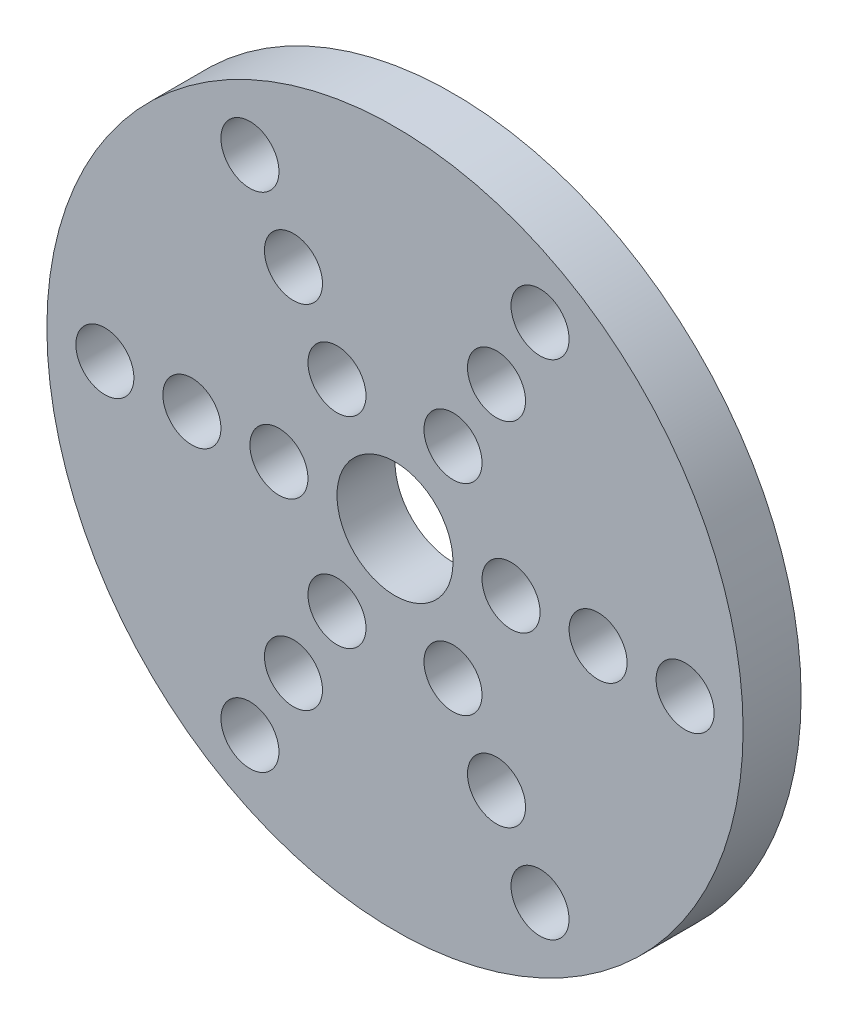
ISO-10303-21;
HEADER;
FILE_DESCRIPTION(('STEP AP214'),'2;1');
FILE_NAME('part.step','',(''),(''),'','','');
FILE_SCHEMA(('AUTOMOTIVE_DESIGN { 1 0 10303 214 1 1 1 1 }'));
ENDSEC;
DATA;
#1=APPLICATION_CONTEXT('core data for automotive mechanical design processes');
#2=APPLICATION_PROTOCOL_DEFINITION('international standard','automotive_design',2000,#1);
#3=PRODUCT_CONTEXT('',#1,'mechanical');
#4=PRODUCT('Part','Part','',(#3));
#5=PRODUCT_RELATED_PRODUCT_CATEGORY('part','',(#4));
#6=PRODUCT_DEFINITION_FORMATION('','',#4);
#7=PRODUCT_DEFINITION_CONTEXT('part definition',#1,'design');
#8=PRODUCT_DEFINITION('design','',#6,#7);
#9=PRODUCT_DEFINITION_SHAPE('','',#8);
#10=(LENGTH_UNIT() NAMED_UNIT(*) SI_UNIT(.MILLI.,.METRE.));
#11=(NAMED_UNIT(*) PLANE_ANGLE_UNIT() SI_UNIT($,.RADIAN.));
#12=(NAMED_UNIT(*) SI_UNIT($,.STERADIAN.) SOLID_ANGLE_UNIT());
#13=UNCERTAINTY_MEASURE_WITH_UNIT(LENGTH_MEASURE(1.E-05),#10,'distance_accuracy_value','');
#14=(GEOMETRIC_REPRESENTATION_CONTEXT(3) GLOBAL_UNCERTAINTY_ASSIGNED_CONTEXT((#13)) GLOBAL_UNIT_ASSIGNED_CONTEXT((#10,
#11,#12)) REPRESENTATION_CONTEXT('',''));
#15=CARTESIAN_POINT('',(0.,0.,0.));
#16=DIRECTION('',(0.,0.,1.));
#17=DIRECTION('',(1.,0.,0.));
#18=AXIS2_PLACEMENT_3D('',#15,#16,#17);
#19=CARTESIAN_POINT('',(0.,0.,10.));
#20=DIRECTION('',(0.,0.,-1.));
#21=DIRECTION('',(-1.,0.,0.));
#22=AXIS2_PLACEMENT_3D('',#19,#20,#21);
#23=CYLINDRICAL_SURFACE('',#22,60.);
#24=CARTESIAN_POINT('',(0.,0.,10.));
#25=DIRECTION('',(0.,0.,1.));
#26=DIRECTION('',(1.,0.,0.));
#27=AXIS2_PLACEMENT_3D('',#24,#25,#26);
#28=CIRCLE('',#27,60.);
#29=CARTESIAN_POINT('',(60.,0.,10.));
#30=VERTEX_POINT('',#29);
#31=EDGE_CURVE('E10',#30,#30,#28,.T.);
#32=ORIENTED_EDGE('',*,*,#31,.F.);
#33=EDGE_LOOP('',(#32));
#34=FACE_BOUND('',#33,.T.);
#35=CARTESIAN_POINT('',(0.,0.,0.));
#36=DIRECTION('',(0.,0.,1.));
#37=DIRECTION('',(1.,0.,0.));
#38=AXIS2_PLACEMENT_3D('',#35,#36,#37);
#39=CIRCLE('',#38,60.);
#40=CARTESIAN_POINT('',(60.,0.,0.));
#41=VERTEX_POINT('',#40);
#42=EDGE_CURVE('E45',#41,#41,#39,.T.);
#43=ORIENTED_EDGE('',*,*,#42,.T.);
#44=EDGE_LOOP('',(#43));
#45=FACE_BOUND('',#44,.T.);
#46=ADVANCED_FACE('F39',(#34,#45),#23,.T.);
#47=CARTESIAN_POINT('',(0.,0.,10.));
#48=DIRECTION('',(0.,0.,1.));
#49=DIRECTION('',(1.,0.,0.));
#50=AXIS2_PLACEMENT_3D('',#47,#48,#49);
#51=PLANE('',#50);
#52=CARTESIAN_POINT('',(17.5000000000004,30.3108891324552,10.));
#53=DIRECTION('',(0.,0.,1.));
#54=DIRECTION('',(0.50000000000001,0.866025403784433,0.));
#55=AXIS2_PLACEMENT_3D('',#52,#53,#54);
#56=CIRCLE('',#55,5.);
#57=CARTESIAN_POINT('',(20.0000000000004,34.6410161513773,10.));
#58=VERTEX_POINT('',#57);
#59=EDGE_CURVE('E157',#58,#58,#56,.T.);
#60=ORIENTED_EDGE('',*,*,#59,.F.);
#61=EDGE_LOOP('',(#60));
#62=FACE_BOUND('',#61,.T.);
#63=CARTESIAN_POINT('',(25.0000000000005,43.3012701892216,10.));
#64=DIRECTION('',(0.,0.,1.));
#65=DIRECTION('',(0.50000000000001,0.866025403784433,0.));
#66=AXIS2_PLACEMENT_3D('',#63,#64,#65);
#67=CIRCLE('',#66,5.);
#68=CARTESIAN_POINT('',(27.5000000000006,47.6313972081438,10.));
#69=VERTEX_POINT('',#68);
#70=EDGE_CURVE('E153',#69,#69,#67,.T.);
#71=ORIENTED_EDGE('',*,*,#70,.F.);
#72=EDGE_LOOP('',(#71));
#73=FACE_BOUND('',#72,.T.);
#74=CARTESIAN_POINT('',(-17.4999999999997,30.3108891324555,10.));
#75=DIRECTION('',(0.,0.,1.));
#76=DIRECTION('',(-0.499999999999992,0.866025403784443,0.));
#77=AXIS2_PLACEMENT_3D('',#74,#75,#76);
#78=CIRCLE('',#77,5.);
#79=CARTESIAN_POINT('',(-19.9999999999997,34.6410161513777,10.));
#80=VERTEX_POINT('',#79);
#81=EDGE_CURVE('E146',#80,#80,#78,.T.);
#82=ORIENTED_EDGE('',*,*,#81,.F.);
#83=EDGE_LOOP('',(#82));
#84=FACE_BOUND('',#83,.T.);
#85=CARTESIAN_POINT('',(-24.9999999999996,43.3012701892222,10.));
#86=DIRECTION('',(0.,0.,1.));
#87=DIRECTION('',(-0.499999999999992,0.866025403784443,0.));
#88=AXIS2_PLACEMENT_3D('',#85,#86,#87);
#89=CIRCLE('',#88,5.);
#90=CARTESIAN_POINT('',(-27.4999999999996,47.6313972081444,10.));
#91=VERTEX_POINT('',#90);
#92=EDGE_CURVE('E143',#91,#91,#89,.T.);
#93=ORIENTED_EDGE('',*,*,#92,.F.);
#94=EDGE_LOOP('',(#93));
#95=FACE_BOUND('',#94,.T.);
#96=CARTESIAN_POINT('',(-35.,0.,10.));
#97=DIRECTION('',(0.,0.,1.));
#98=DIRECTION('',(-1.,0.,0.));
#99=AXIS2_PLACEMENT_3D('',#96,#97,#98);
#100=CIRCLE('',#99,5.);
#101=CARTESIAN_POINT('',(-40.,0.,10.));
#102=VERTEX_POINT('',#101);
#103=EDGE_CURVE('E138',#102,#102,#100,.T.);
#104=ORIENTED_EDGE('',*,*,#103,.F.);
#105=EDGE_LOOP('',(#104));
#106=FACE_BOUND('',#105,.T.);
#107=CARTESIAN_POINT('',(-50.,0.,10.));
#108=DIRECTION('',(0.,0.,1.));
#109=DIRECTION('',(-1.,0.,0.));
#110=AXIS2_PLACEMENT_3D('',#107,#108,#109);
#111=CIRCLE('',#110,5.);
#112=CARTESIAN_POINT('',(-55.,0.,10.));
#113=VERTEX_POINT('',#112);
#114=EDGE_CURVE('E129',#113,#113,#111,.T.);
#115=ORIENTED_EDGE('',*,*,#114,.F.);
#116=EDGE_LOOP('',(#115));
#117=FACE_BOUND('',#116,.T.);
#118=CARTESIAN_POINT('',(-17.5000000000001,-30.3108891324553,10.));
#119=DIRECTION('',(0.,0.,1.));
#120=DIRECTION('',(-0.500000000000004,-0.866025403784436,0.));
#121=AXIS2_PLACEMENT_3D('',#118,#119,#120);
#122=CIRCLE('',#121,5.);
#123=CARTESIAN_POINT('',(-20.0000000000002,-34.6410161513775,10.));
#124=VERTEX_POINT('',#123);
#125=EDGE_CURVE('E122',#124,#124,#122,.T.);
#126=ORIENTED_EDGE('',*,*,#125,.F.);
#127=EDGE_LOOP('',(#126));
#128=FACE_BOUND('',#127,.T.);
#129=CARTESIAN_POINT('',(-25.0000000000002,-43.3012701892218,10.));
#130=DIRECTION('',(0.,0.,1.));
#131=DIRECTION('',(-0.500000000000004,-0.866025403784436,0.));
#132=AXIS2_PLACEMENT_3D('',#129,#130,#131);
#133=CIRCLE('',#132,5.);
#134=CARTESIAN_POINT('',(-27.5000000000002,-47.631397208144,10.));
#135=VERTEX_POINT('',#134);
#136=EDGE_CURVE('E119',#135,#135,#133,.T.);
#137=ORIENTED_EDGE('',*,*,#136,.F.);
#138=EDGE_LOOP('',(#137));
#139=FACE_BOUND('',#138,.T.);
#140=CARTESIAN_POINT('',(17.4999999999999,-30.3108891324554,10.));
#141=DIRECTION('',(0.,0.,1.));
#142=DIRECTION('',(0.499999999999998,-0.86602540378444,0.));
#143=AXIS2_PLACEMENT_3D('',#140,#141,#142);
#144=CIRCLE('',#143,5.);
#145=CARTESIAN_POINT('',(19.9999999999999,-34.6410161513776,10.));
#146=VERTEX_POINT('',#145);
#147=EDGE_CURVE('E115',#146,#146,#144,.T.);
#148=ORIENTED_EDGE('',*,*,#147,.F.);
#149=EDGE_LOOP('',(#148));
#150=FACE_BOUND('',#149,.T.);
#151=CARTESIAN_POINT('',(24.9999999999999,-43.301270189222,10.));
#152=DIRECTION('',(0.,0.,1.));
#153=DIRECTION('',(0.499999999999998,-0.86602540378444,0.));
#154=AXIS2_PLACEMENT_3D('',#151,#152,#153);
#155=CIRCLE('',#154,5.);
#156=CARTESIAN_POINT('',(27.4999999999999,-47.6313972081442,10.));
#157=VERTEX_POINT('',#156);
#158=EDGE_CURVE('E104',#157,#157,#155,.T.);
#159=ORIENTED_EDGE('',*,*,#158,.F.);
#160=EDGE_LOOP('',(#159));
#161=FACE_BOUND('',#160,.T.);
#162=CARTESIAN_POINT('',(35.,0.,10.));
#163=DIRECTION('',(0.,0.,1.));
#164=DIRECTION('',(1.,0.,0.));
#165=AXIS2_PLACEMENT_3D('',#162,#163,#164);
#166=CIRCLE('',#165,5.);
#167=CARTESIAN_POINT('',(40.,0.,10.));
#168=VERTEX_POINT('',#167);
#169=EDGE_CURVE('E99',#168,#168,#166,.T.);
#170=ORIENTED_EDGE('',*,*,#169,.F.);
#171=EDGE_LOOP('',(#170));
#172=FACE_BOUND('',#171,.T.);
#173=CARTESIAN_POINT('',(50.,0.,10.));
#174=DIRECTION('',(0.,0.,1.));
#175=DIRECTION('',(1.,0.,0.));
#176=AXIS2_PLACEMENT_3D('',#173,#174,#175);
#177=CIRCLE('',#176,5.);
#178=CARTESIAN_POINT('',(55.,0.,10.));
#179=VERTEX_POINT('',#178);
#180=EDGE_CURVE('E91',#179,#179,#177,.T.);
#181=ORIENTED_EDGE('',*,*,#180,.F.);
#182=EDGE_LOOP('',(#181));
#183=FACE_BOUND('',#182,.T.);
#184=CARTESIAN_POINT('',(10.0000000000002,17.3205080756887,10.));
#185=DIRECTION('',(0.,0.,1.));
#186=DIRECTION('',(0.50000000000001,0.866025403784433,0.));
#187=AXIS2_PLACEMENT_3D('',#184,#185,#186);
#188=CIRCLE('',#187,5.);
#189=CARTESIAN_POINT('',(12.5000000000003,21.6506350946108,10.));
#190=VERTEX_POINT('',#189);
#191=EDGE_CURVE('E67',#190,#190,#188,.T.);
#192=ORIENTED_EDGE('',*,*,#191,.F.);
#193=EDGE_LOOP('',(#192));
#194=FACE_BOUND('',#193,.T.);
#195=CARTESIAN_POINT('',(-9.99999999999984,17.3205080756889,10.));
#196=DIRECTION('',(0.,0.,1.));
#197=DIRECTION('',(-0.499999999999992,0.866025403784443,0.));
#198=AXIS2_PLACEMENT_3D('',#195,#196,#197);
#199=CIRCLE('',#198,5.);
#200=CARTESIAN_POINT('',(-12.4999999999998,21.6506350946111,10.));
#201=VERTEX_POINT('',#200);
#202=EDGE_CURVE('E78',#201,#201,#199,.T.);
#203=ORIENTED_EDGE('',*,*,#202,.F.);
#204=EDGE_LOOP('',(#203));
#205=FACE_BOUND('',#204,.T.);
#206=CARTESIAN_POINT('',(-20.,0.,10.));
#207=DIRECTION('',(0.,0.,1.));
#208=DIRECTION('',(-1.,0.,0.));
#209=AXIS2_PLACEMENT_3D('',#206,#207,#208);
#210=CIRCLE('',#209,5.);
#211=CARTESIAN_POINT('',(-25.,0.,10.));
#212=VERTEX_POINT('',#211);
#213=EDGE_CURVE('E85',#212,#212,#210,.T.);
#214=ORIENTED_EDGE('',*,*,#213,.F.);
#215=EDGE_LOOP('',(#214));
#216=FACE_BOUND('',#215,.T.);
#217=CARTESIAN_POINT('',(-10.0000000000001,-17.3205080756887,10.));
#218=DIRECTION('',(0.,0.,1.));
#219=DIRECTION('',(-0.500000000000004,-0.866025403784436,0.));
#220=AXIS2_PLACEMENT_3D('',#217,#218,#219);
#221=CIRCLE('',#220,5.);
#222=CARTESIAN_POINT('',(-12.5000000000001,-21.6506350946109,10.));
#223=VERTEX_POINT('',#222);
#224=EDGE_CURVE('E86',#223,#223,#221,.T.);
#225=ORIENTED_EDGE('',*,*,#224,.F.);
#226=EDGE_LOOP('',(#225));
#227=FACE_BOUND('',#226,.T.);
#228=CARTESIAN_POINT('',(9.99999999999996,-17.3205080756888,10.));
#229=DIRECTION('',(0.,0.,1.));
#230=DIRECTION('',(0.499999999999998,-0.86602540378444,0.));
#231=AXIS2_PLACEMENT_3D('',#228,#229,#230);
#232=CIRCLE('',#231,5.);
#233=CARTESIAN_POINT('',(12.5,-21.650635094611,10.));
#234=VERTEX_POINT('',#233);
#235=EDGE_CURVE('E62',#234,#234,#232,.T.);
#236=ORIENTED_EDGE('',*,*,#235,.F.);
#237=EDGE_LOOP('',(#236));
#238=FACE_BOUND('',#237,.T.);
#239=CARTESIAN_POINT('',(20.,0.,10.));
#240=DIRECTION('',(0.,0.,1.));
#241=DIRECTION('',(1.,0.,0.));
#242=AXIS2_PLACEMENT_3D('',#239,#240,#241);
#243=CIRCLE('',#242,5.);
#244=CARTESIAN_POINT('',(25.,0.,10.));
#245=VERTEX_POINT('',#244);
#246=EDGE_CURVE('E60',#245,#245,#243,.T.);
#247=ORIENTED_EDGE('',*,*,#246,.F.);
#248=EDGE_LOOP('',(#247));
#249=FACE_BOUND('',#248,.T.);
#250=CARTESIAN_POINT('',(0.,0.,10.));
#251=DIRECTION('',(0.,0.,1.));
#252=DIRECTION('',(1.,0.,0.));
#253=AXIS2_PLACEMENT_3D('',#250,#251,#252);
#254=CIRCLE('',#253,10.);
#255=CARTESIAN_POINT('',(10.,0.,10.));
#256=VERTEX_POINT('',#255);
#257=EDGE_CURVE('E51',#256,#256,#254,.T.);
#258=ORIENTED_EDGE('',*,*,#257,.F.);
#259=EDGE_LOOP('',(#258));
#260=FACE_BOUND('',#259,.T.);
#261=ORIENTED_EDGE('',*,*,#31,.T.);
#262=EDGE_LOOP('',(#261));
#263=FACE_BOUND('',#262,.T.);
#264=ADVANCED_FACE('F171',(#62,#73,#84,#95,#106,#117,#128,#139,#150,#161,#172,#183,#194,#205,
#216,#227,#238,#249,#260,#263),#51,.T.);
#265=CARTESIAN_POINT('',(0.,0.,0.));
#266=DIRECTION('',(0.,0.,1.));
#267=DIRECTION('',(1.,0.,0.));
#268=AXIS2_PLACEMENT_3D('',#265,#266,#267);
#269=PLANE('',#268);
#270=CARTESIAN_POINT('',(17.5000000000004,30.3108891324552,0.));
#271=DIRECTION('',(0.,0.,1.));
#272=DIRECTION('',(0.50000000000001,0.866025403784433,0.));
#273=AXIS2_PLACEMENT_3D('',#270,#271,#272);
#274=CIRCLE('',#273,5.);
#275=CARTESIAN_POINT('',(20.0000000000004,34.6410161513773,0.));
#276=VERTEX_POINT('',#275);
#277=EDGE_CURVE('E144',#276,#276,#274,.T.);
#278=ORIENTED_EDGE('',*,*,#277,.T.);
#279=EDGE_LOOP('',(#278));
#280=FACE_BOUND('',#279,.T.);
#281=CARTESIAN_POINT('',(25.0000000000005,43.3012701892216,0.));
#282=DIRECTION('',(0.,0.,1.));
#283=DIRECTION('',(0.50000000000001,0.866025403784433,0.));
#284=AXIS2_PLACEMENT_3D('',#281,#282,#283);
#285=CIRCLE('',#284,5.);
#286=CARTESIAN_POINT('',(27.5000000000006,47.6313972081438,0.));
#287=VERTEX_POINT('',#286);
#288=EDGE_CURVE('E156',#287,#287,#285,.T.);
#289=ORIENTED_EDGE('',*,*,#288,.T.);
#290=EDGE_LOOP('',(#289));
#291=FACE_BOUND('',#290,.T.);
#292=CARTESIAN_POINT('',(-17.4999999999997,30.3108891324555,0.));
#293=DIRECTION('',(0.,0.,1.));
#294=DIRECTION('',(-0.499999999999992,0.866025403784443,0.));
#295=AXIS2_PLACEMENT_3D('',#292,#293,#294);
#296=CIRCLE('',#295,5.);
#297=CARTESIAN_POINT('',(-19.9999999999997,34.6410161513777,0.));
#298=VERTEX_POINT('',#297);
#299=EDGE_CURVE('E132',#298,#298,#296,.T.);
#300=ORIENTED_EDGE('',*,*,#299,.T.);
#301=EDGE_LOOP('',(#300));
#302=FACE_BOUND('',#301,.T.);
#303=CARTESIAN_POINT('',(-24.9999999999996,43.3012701892222,0.));
#304=DIRECTION('',(0.,0.,1.));
#305=DIRECTION('',(-0.499999999999992,0.866025403784443,0.));
#306=AXIS2_PLACEMENT_3D('',#303,#304,#305);
#307=CIRCLE('',#306,5.);
#308=CARTESIAN_POINT('',(-27.4999999999996,47.6313972081444,0.));
#309=VERTEX_POINT('',#308);
#310=EDGE_CURVE('E145',#309,#309,#307,.T.);
#311=ORIENTED_EDGE('',*,*,#310,.T.);
#312=EDGE_LOOP('',(#311));
#313=FACE_BOUND('',#312,.T.);
#314=CARTESIAN_POINT('',(-35.,0.,0.));
#315=DIRECTION('',(0.,0.,1.));
#316=DIRECTION('',(-1.,0.,0.));
#317=AXIS2_PLACEMENT_3D('',#314,#315,#316);
#318=CIRCLE('',#317,5.);
#319=CARTESIAN_POINT('',(-40.,0.,0.));
#320=VERTEX_POINT('',#319);
#321=EDGE_CURVE('E123',#320,#320,#318,.T.);
#322=ORIENTED_EDGE('',*,*,#321,.T.);
#323=EDGE_LOOP('',(#322));
#324=FACE_BOUND('',#323,.T.);
#325=CARTESIAN_POINT('',(-50.,0.,0.));
#326=DIRECTION('',(0.,0.,1.));
#327=DIRECTION('',(-1.,0.,0.));
#328=AXIS2_PLACEMENT_3D('',#325,#326,#327);
#329=CIRCLE('',#328,5.);
#330=CARTESIAN_POINT('',(-55.,0.,0.));
#331=VERTEX_POINT('',#330);
#332=EDGE_CURVE('E134',#331,#331,#329,.T.);
#333=ORIENTED_EDGE('',*,*,#332,.T.);
#334=EDGE_LOOP('',(#333));
#335=FACE_BOUND('',#334,.T.);
#336=CARTESIAN_POINT('',(-17.5000000000001,-30.3108891324553,0.));
#337=DIRECTION('',(0.,0.,1.));
#338=DIRECTION('',(-0.500000000000004,-0.866025403784436,0.));
#339=AXIS2_PLACEMENT_3D('',#336,#337,#338);
#340=CIRCLE('',#339,5.);
#341=CARTESIAN_POINT('',(-20.0000000000002,-34.6410161513775,0.));
#342=VERTEX_POINT('',#341);
#343=EDGE_CURVE('E108',#342,#342,#340,.T.);
#344=ORIENTED_EDGE('',*,*,#343,.T.);
#345=EDGE_LOOP('',(#344));
#346=FACE_BOUND('',#345,.T.);
#347=CARTESIAN_POINT('',(-25.0000000000002,-43.3012701892218,0.));
#348=DIRECTION('',(0.,0.,1.));
#349=DIRECTION('',(-0.500000000000004,-0.866025403784436,0.));
#350=AXIS2_PLACEMENT_3D('',#347,#348,#349);
#351=CIRCLE('',#350,5.);
#352=CARTESIAN_POINT('',(-27.5000000000002,-47.631397208144,0.));
#353=VERTEX_POINT('',#352);
#354=EDGE_CURVE('E116',#353,#353,#351,.T.);
#355=ORIENTED_EDGE('',*,*,#354,.T.);
#356=EDGE_LOOP('',(#355));
#357=FACE_BOUND('',#356,.T.);
#358=CARTESIAN_POINT('',(17.4999999999999,-30.3108891324554,0.));
#359=DIRECTION('',(0.,0.,1.));
#360=DIRECTION('',(0.499999999999998,-0.86602540378444,0.));
#361=AXIS2_PLACEMENT_3D('',#358,#359,#360);
#362=CIRCLE('',#361,5.);
#363=CARTESIAN_POINT('',(19.9999999999999,-34.6410161513776,0.));
#364=VERTEX_POINT('',#363);
#365=EDGE_CURVE('E100',#364,#364,#362,.T.);
#366=ORIENTED_EDGE('',*,*,#365,.T.);
#367=EDGE_LOOP('',(#366));
#368=FACE_BOUND('',#367,.T.);
#369=CARTESIAN_POINT('',(24.9999999999999,-43.301270189222,0.));
#370=DIRECTION('',(0.,0.,1.));
#371=DIRECTION('',(0.499999999999998,-0.86602540378444,0.));
#372=AXIS2_PLACEMENT_3D('',#369,#370,#371);
#373=CIRCLE('',#372,5.);
#374=CARTESIAN_POINT('',(27.4999999999999,-47.6313972081442,0.));
#375=VERTEX_POINT('',#374);
#376=EDGE_CURVE('E107',#375,#375,#373,.T.);
#377=ORIENTED_EDGE('',*,*,#376,.T.);
#378=EDGE_LOOP('',(#377));
#379=FACE_BOUND('',#378,.T.);
#380=CARTESIAN_POINT('',(35.,0.,0.));
#381=DIRECTION('',(0.,0.,1.));
#382=DIRECTION('',(1.,0.,0.));
#383=AXIS2_PLACEMENT_3D('',#380,#381,#382);
#384=CIRCLE('',#383,5.);
#385=CARTESIAN_POINT('',(40.,0.,0.));
#386=VERTEX_POINT('',#385);
#387=EDGE_CURVE('E71',#386,#386,#384,.T.);
#388=ORIENTED_EDGE('',*,*,#387,.T.);
#389=EDGE_LOOP('',(#388));
#390=FACE_BOUND('',#389,.T.);
#391=CARTESIAN_POINT('',(50.,0.,0.));
#392=DIRECTION('',(0.,0.,1.));
#393=DIRECTION('',(1.,0.,0.));
#394=AXIS2_PLACEMENT_3D('',#391,#392,#393);
#395=CIRCLE('',#394,5.);
#396=CARTESIAN_POINT('',(55.,0.,0.));
#397=VERTEX_POINT('',#396);
#398=EDGE_CURVE('E96',#397,#397,#395,.T.);
#399=ORIENTED_EDGE('',*,*,#398,.T.);
#400=EDGE_LOOP('',(#399));
#401=FACE_BOUND('',#400,.T.);
#402=CARTESIAN_POINT('',(10.0000000000002,17.3205080756887,0.));
#403=DIRECTION('',(0.,0.,1.));
#404=DIRECTION('',(0.50000000000001,0.866025403784433,0.));
#405=AXIS2_PLACEMENT_3D('',#402,#403,#404);
#406=CIRCLE('',#405,5.);
#407=CARTESIAN_POINT('',(12.5000000000003,21.6506350946108,0.));
#408=VERTEX_POINT('',#407);
#409=EDGE_CURVE('E75',#408,#408,#406,.T.);
#410=ORIENTED_EDGE('',*,*,#409,.T.);
#411=EDGE_LOOP('',(#410));
#412=FACE_BOUND('',#411,.T.);
#413=CARTESIAN_POINT('',(-9.99999999999984,17.3205080756889,0.));
#414=DIRECTION('',(0.,0.,1.));
#415=DIRECTION('',(-0.499999999999992,0.866025403784443,0.));
#416=AXIS2_PLACEMENT_3D('',#413,#414,#415);
#417=CIRCLE('',#416,5.);
#418=CARTESIAN_POINT('',(-12.4999999999998,21.6506350946111,0.));
#419=VERTEX_POINT('',#418);
#420=EDGE_CURVE('E80',#419,#419,#417,.T.);
#421=ORIENTED_EDGE('',*,*,#420,.T.);
#422=EDGE_LOOP('',(#421));
#423=FACE_BOUND('',#422,.T.);
#424=CARTESIAN_POINT('',(-20.,0.,0.));
#425=DIRECTION('',(0.,0.,1.));
#426=DIRECTION('',(-1.,0.,0.));
#427=AXIS2_PLACEMENT_3D('',#424,#425,#426);
#428=CIRCLE('',#427,5.);
#429=CARTESIAN_POINT('',(-25.,0.,0.));
#430=VERTEX_POINT('',#429);
#431=EDGE_CURVE('E84',#430,#430,#428,.T.);
#432=ORIENTED_EDGE('',*,*,#431,.T.);
#433=EDGE_LOOP('',(#432));
#434=FACE_BOUND('',#433,.T.);
#435=CARTESIAN_POINT('',(-10.0000000000001,-17.3205080756887,0.));
#436=DIRECTION('',(0.,0.,1.));
#437=DIRECTION('',(-0.500000000000004,-0.866025403784436,0.));
#438=AXIS2_PLACEMENT_3D('',#435,#436,#437);
#439=CIRCLE('',#438,5.);
#440=CARTESIAN_POINT('',(-12.5000000000001,-21.6506350946109,0.));
#441=VERTEX_POINT('',#440);
#442=EDGE_CURVE('E68',#441,#441,#439,.T.);
#443=ORIENTED_EDGE('',*,*,#442,.T.);
#444=EDGE_LOOP('',(#443));
#445=FACE_BOUND('',#444,.T.);
#446=CARTESIAN_POINT('',(9.99999999999996,-17.3205080756888,0.));
#447=DIRECTION('',(0.,0.,1.));
#448=DIRECTION('',(0.499999999999998,-0.86602540378444,0.));
#449=AXIS2_PLACEMENT_3D('',#446,#447,#448);
#450=CIRCLE('',#449,5.);
#451=CARTESIAN_POINT('',(12.5,-21.650635094611,0.));
#452=VERTEX_POINT('',#451);
#453=EDGE_CURVE('E58',#452,#452,#450,.T.);
#454=ORIENTED_EDGE('',*,*,#453,.T.);
#455=EDGE_LOOP('',(#454));
#456=FACE_BOUND('',#455,.T.);
#457=CARTESIAN_POINT('',(20.,0.,0.));
#458=DIRECTION('',(0.,0.,1.));
#459=DIRECTION('',(1.,0.,0.));
#460=AXIS2_PLACEMENT_3D('',#457,#458,#459);
#461=CIRCLE('',#460,5.);
#462=CARTESIAN_POINT('',(25.,0.,0.));
#463=VERTEX_POINT('',#462);
#464=EDGE_CURVE('E53',#463,#463,#461,.T.);
#465=ORIENTED_EDGE('',*,*,#464,.T.);
#466=EDGE_LOOP('',(#465));
#467=FACE_BOUND('',#466,.T.);
#468=CARTESIAN_POINT('',(0.,0.,0.));
#469=DIRECTION('',(0.,0.,1.));
#470=DIRECTION('',(1.,0.,0.));
#471=AXIS2_PLACEMENT_3D('',#468,#469,#470);
#472=CIRCLE('',#471,10.);
#473=CARTESIAN_POINT('',(10.,0.,0.));
#474=VERTEX_POINT('',#473);
#475=EDGE_CURVE('E47',#474,#474,#472,.T.);
#476=ORIENTED_EDGE('',*,*,#475,.T.);
#477=EDGE_LOOP('',(#476));
#478=FACE_BOUND('',#477,.T.);
#479=ORIENTED_EDGE('',*,*,#42,.F.);
#480=EDGE_LOOP('',(#479));
#481=FACE_BOUND('',#480,.T.);
#482=ADVANCED_FACE('F164',(#280,#291,#302,#313,#324,#335,#346,#357,#368,#379,#390,#401,#412,
#423,#434,#445,#456,#467,#478,#481),#269,.F.);
#483=CARTESIAN_POINT('',(0.,0.,0.));
#484=DIRECTION('',(0.,0.,1.));
#485=DIRECTION('',(1.,0.,0.));
#486=AXIS2_PLACEMENT_3D('',#483,#484,#485);
#487=CYLINDRICAL_SURFACE('',#486,10.);
#488=ORIENTED_EDGE('',*,*,#475,.F.);
#489=EDGE_LOOP('',(#488));
#490=FACE_BOUND('',#489,.T.);
#491=ORIENTED_EDGE('',*,*,#257,.T.);
#492=EDGE_LOOP('',(#491));
#493=FACE_BOUND('',#492,.T.);
#494=ADVANCED_FACE('F214',(#490,#493),#487,.F.);
#495=CARTESIAN_POINT('',(20.,0.,0.));
#496=DIRECTION('',(0.,0.,1.));
#497=DIRECTION('',(1.,0.,0.));
#498=AXIS2_PLACEMENT_3D('',#495,#496,#497);
#499=CYLINDRICAL_SURFACE('',#498,5.);
#500=ORIENTED_EDGE('',*,*,#464,.F.);
#501=EDGE_LOOP('',(#500));
#502=FACE_BOUND('',#501,.T.);
#503=ORIENTED_EDGE('',*,*,#246,.T.);
#504=EDGE_LOOP('',(#503));
#505=FACE_BOUND('',#504,.T.);
#506=ADVANCED_FACE('F220',(#502,#505),#499,.F.);
#507=CARTESIAN_POINT('',(9.99999999999996,-17.3205080756888,0.));
#508=DIRECTION('',(0.,0.,1.));
#509=DIRECTION('',(1.,0.,0.));
#510=AXIS2_PLACEMENT_3D('',#507,#508,#509);
#511=CYLINDRICAL_SURFACE('',#510,5.);
#512=ORIENTED_EDGE('',*,*,#453,.F.);
#513=EDGE_LOOP('',(#512));
#514=FACE_BOUND('',#513,.T.);
#515=ORIENTED_EDGE('',*,*,#235,.T.);
#516=EDGE_LOOP('',(#515));
#517=FACE_BOUND('',#516,.T.);
#518=ADVANCED_FACE('F221',(#514,#517),#511,.F.);
#519=CARTESIAN_POINT('',(-10.0000000000001,-17.3205080756887,0.));
#520=DIRECTION('',(0.,0.,1.));
#521=DIRECTION('',(1.,0.,0.));
#522=AXIS2_PLACEMENT_3D('',#519,#520,#521);
#523=CYLINDRICAL_SURFACE('',#522,5.);
#524=ORIENTED_EDGE('',*,*,#442,.F.);
#525=EDGE_LOOP('',(#524));
#526=FACE_BOUND('',#525,.T.);
#527=ORIENTED_EDGE('',*,*,#224,.T.);
#528=EDGE_LOOP('',(#527));
#529=FACE_BOUND('',#528,.T.);
#530=ADVANCED_FACE('F268',(#526,#529),#523,.F.);
#531=CARTESIAN_POINT('',(-20.,0.,0.));
#532=DIRECTION('',(0.,0.,1.));
#533=DIRECTION('',(1.,0.,0.));
#534=AXIS2_PLACEMENT_3D('',#531,#532,#533);
#535=CYLINDRICAL_SURFACE('',#534,5.);
#536=ORIENTED_EDGE('',*,*,#431,.F.);
#537=EDGE_LOOP('',(#536));
#538=FACE_BOUND('',#537,.T.);
#539=ORIENTED_EDGE('',*,*,#213,.T.);
#540=EDGE_LOOP('',(#539));
#541=FACE_BOUND('',#540,.T.);
#542=ADVANCED_FACE('F279',(#538,#541),#535,.F.);
#543=CARTESIAN_POINT('',(-9.99999999999984,17.3205080756889,0.));
#544=DIRECTION('',(0.,0.,1.));
#545=DIRECTION('',(1.,0.,0.));
#546=AXIS2_PLACEMENT_3D('',#543,#544,#545);
#547=CYLINDRICAL_SURFACE('',#546,5.);
#548=ORIENTED_EDGE('',*,*,#420,.F.);
#549=EDGE_LOOP('',(#548));
#550=FACE_BOUND('',#549,.T.);
#551=ORIENTED_EDGE('',*,*,#202,.T.);
#552=EDGE_LOOP('',(#551));
#553=FACE_BOUND('',#552,.T.);
#554=ADVANCED_FACE('F286',(#550,#553),#547,.F.);
#555=CARTESIAN_POINT('',(10.0000000000002,17.3205080756887,0.));
#556=DIRECTION('',(0.,0.,1.));
#557=DIRECTION('',(1.,0.,0.));
#558=AXIS2_PLACEMENT_3D('',#555,#556,#557);
#559=CYLINDRICAL_SURFACE('',#558,5.);
#560=ORIENTED_EDGE('',*,*,#409,.F.);
#561=EDGE_LOOP('',(#560));
#562=FACE_BOUND('',#561,.T.);
#563=ORIENTED_EDGE('',*,*,#191,.T.);
#564=EDGE_LOOP('',(#563));
#565=FACE_BOUND('',#564,.T.);
#566=ADVANCED_FACE('F297',(#562,#565),#559,.F.);
#567=CARTESIAN_POINT('',(50.,0.,0.));
#568=DIRECTION('',(0.,0.,1.));
#569=DIRECTION('',(1.,0.,0.));
#570=AXIS2_PLACEMENT_3D('',#567,#568,#569);
#571=CYLINDRICAL_SURFACE('',#570,5.);
#572=ORIENTED_EDGE('',*,*,#398,.F.);
#573=EDGE_LOOP('',(#572));
#574=FACE_BOUND('',#573,.T.);
#575=ORIENTED_EDGE('',*,*,#180,.T.);
#576=EDGE_LOOP('',(#575));
#577=FACE_BOUND('',#576,.T.);
#578=ADVANCED_FACE('F306',(#574,#577),#571,.F.);
#579=CARTESIAN_POINT('',(35.,0.,0.));
#580=DIRECTION('',(0.,0.,1.));
#581=DIRECTION('',(1.,0.,0.));
#582=AXIS2_PLACEMENT_3D('',#579,#580,#581);
#583=CYLINDRICAL_SURFACE('',#582,5.);
#584=ORIENTED_EDGE('',*,*,#387,.F.);
#585=EDGE_LOOP('',(#584));
#586=FACE_BOUND('',#585,.T.);
#587=ORIENTED_EDGE('',*,*,#169,.T.);
#588=EDGE_LOOP('',(#587));
#589=FACE_BOUND('',#588,.T.);
#590=ADVANCED_FACE('F318',(#586,#589),#583,.F.);
#591=CARTESIAN_POINT('',(24.9999999999999,-43.301270189222,0.));
#592=DIRECTION('',(0.,0.,1.));
#593=DIRECTION('',(1.,0.,0.));
#594=AXIS2_PLACEMENT_3D('',#591,#592,#593);
#595=CYLINDRICAL_SURFACE('',#594,5.);
#596=ORIENTED_EDGE('',*,*,#376,.F.);
#597=EDGE_LOOP('',(#596));
#598=FACE_BOUND('',#597,.T.);
#599=ORIENTED_EDGE('',*,*,#158,.T.);
#600=EDGE_LOOP('',(#599));
#601=FACE_BOUND('',#600,.T.);
#602=ADVANCED_FACE('F327',(#598,#601),#595,.F.);
#603=CARTESIAN_POINT('',(17.4999999999999,-30.3108891324554,0.));
#604=DIRECTION('',(0.,0.,1.));
#605=DIRECTION('',(1.,0.,0.));
#606=AXIS2_PLACEMENT_3D('',#603,#604,#605);
#607=CYLINDRICAL_SURFACE('',#606,5.);
#608=ORIENTED_EDGE('',*,*,#365,.F.);
#609=EDGE_LOOP('',(#608));
#610=FACE_BOUND('',#609,.T.);
#611=ORIENTED_EDGE('',*,*,#147,.T.);
#612=EDGE_LOOP('',(#611));
#613=FACE_BOUND('',#612,.T.);
#614=ADVANCED_FACE('F339',(#610,#613),#607,.F.);
#615=CARTESIAN_POINT('',(-25.0000000000002,-43.3012701892218,0.));
#616=DIRECTION('',(0.,0.,1.));
#617=DIRECTION('',(1.,0.,0.));
#618=AXIS2_PLACEMENT_3D('',#615,#616,#617);
#619=CYLINDRICAL_SURFACE('',#618,5.);
#620=ORIENTED_EDGE('',*,*,#354,.F.);
#621=EDGE_LOOP('',(#620));
#622=FACE_BOUND('',#621,.T.);
#623=ORIENTED_EDGE('',*,*,#136,.T.);
#624=EDGE_LOOP('',(#623));
#625=FACE_BOUND('',#624,.T.);
#626=ADVANCED_FACE('F350',(#622,#625),#619,.F.);
#627=CARTESIAN_POINT('',(-17.5000000000001,-30.3108891324553,0.));
#628=DIRECTION('',(0.,0.,1.));
#629=DIRECTION('',(1.,0.,0.));
#630=AXIS2_PLACEMENT_3D('',#627,#628,#629);
#631=CYLINDRICAL_SURFACE('',#630,5.);
#632=ORIENTED_EDGE('',*,*,#343,.F.);
#633=EDGE_LOOP('',(#632));
#634=FACE_BOUND('',#633,.T.);
#635=ORIENTED_EDGE('',*,*,#125,.T.);
#636=EDGE_LOOP('',(#635));
#637=FACE_BOUND('',#636,.T.);
#638=ADVANCED_FACE('F360',(#634,#637),#631,.F.);
#639=CARTESIAN_POINT('',(-50.,0.,0.));
#640=DIRECTION('',(0.,0.,1.));
#641=DIRECTION('',(1.,0.,0.));
#642=AXIS2_PLACEMENT_3D('',#639,#640,#641);
#643=CYLINDRICAL_SURFACE('',#642,5.);
#644=ORIENTED_EDGE('',*,*,#332,.F.);
#645=EDGE_LOOP('',(#644));
#646=FACE_BOUND('',#645,.T.);
#647=ORIENTED_EDGE('',*,*,#114,.T.);
#648=EDGE_LOOP('',(#647));
#649=FACE_BOUND('',#648,.T.);
#650=ADVANCED_FACE('F370',(#646,#649),#643,.F.);
#651=CARTESIAN_POINT('',(-35.,0.,0.));
#652=DIRECTION('',(0.,0.,1.));
#653=DIRECTION('',(1.,0.,0.));
#654=AXIS2_PLACEMENT_3D('',#651,#652,#653);
#655=CYLINDRICAL_SURFACE('',#654,5.);
#656=ORIENTED_EDGE('',*,*,#321,.F.);
#657=EDGE_LOOP('',(#656));
#658=FACE_BOUND('',#657,.T.);
#659=ORIENTED_EDGE('',*,*,#103,.T.);
#660=EDGE_LOOP('',(#659));
#661=FACE_BOUND('',#660,.T.);
#662=ADVANCED_FACE('F380',(#658,#661),#655,.F.);
#663=CARTESIAN_POINT('',(-24.9999999999996,43.3012701892222,0.));
#664=DIRECTION('',(0.,0.,1.));
#665=DIRECTION('',(1.,0.,0.));
#666=AXIS2_PLACEMENT_3D('',#663,#664,#665);
#667=CYLINDRICAL_SURFACE('',#666,5.);
#668=ORIENTED_EDGE('',*,*,#310,.F.);
#669=EDGE_LOOP('',(#668));
#670=FACE_BOUND('',#669,.T.);
#671=ORIENTED_EDGE('',*,*,#92,.T.);
#672=EDGE_LOOP('',(#671));
#673=FACE_BOUND('',#672,.T.);
#674=ADVANCED_FACE('F390',(#670,#673),#667,.F.);
#675=CARTESIAN_POINT('',(-17.4999999999997,30.3108891324555,0.));
#676=DIRECTION('',(0.,0.,1.));
#677=DIRECTION('',(1.,0.,0.));
#678=AXIS2_PLACEMENT_3D('',#675,#676,#677);
#679=CYLINDRICAL_SURFACE('',#678,5.);
#680=ORIENTED_EDGE('',*,*,#299,.F.);
#681=EDGE_LOOP('',(#680));
#682=FACE_BOUND('',#681,.T.);
#683=ORIENTED_EDGE('',*,*,#81,.T.);
#684=EDGE_LOOP('',(#683));
#685=FACE_BOUND('',#684,.T.);
#686=ADVANCED_FACE('F400',(#682,#685),#679,.F.);
#687=CARTESIAN_POINT('',(25.0000000000005,43.3012701892216,0.));
#688=DIRECTION('',(0.,0.,1.));
#689=DIRECTION('',(1.,0.,0.));
#690=AXIS2_PLACEMENT_3D('',#687,#688,#689);
#691=CYLINDRICAL_SURFACE('',#690,5.);
#692=ORIENTED_EDGE('',*,*,#288,.F.);
#693=EDGE_LOOP('',(#692));
#694=FACE_BOUND('',#693,.T.);
#695=ORIENTED_EDGE('',*,*,#70,.T.);
#696=EDGE_LOOP('',(#695));
#697=FACE_BOUND('',#696,.T.);
#698=ADVANCED_FACE('F173',(#694,#697),#691,.F.);
#699=CARTESIAN_POINT('',(17.5000000000004,30.3108891324552,0.));
#700=DIRECTION('',(0.,0.,1.));
#701=DIRECTION('',(1.,0.,0.));
#702=AXIS2_PLACEMENT_3D('',#699,#700,#701);
#703=CYLINDRICAL_SURFACE('',#702,5.);
#704=ORIENTED_EDGE('',*,*,#277,.F.);
#705=EDGE_LOOP('',(#704));
#706=FACE_BOUND('',#705,.T.);
#707=ORIENTED_EDGE('',*,*,#59,.T.);
#708=EDGE_LOOP('',(#707));
#709=FACE_BOUND('',#708,.T.);
#710=ADVANCED_FACE('F169',(#706,#709),#703,.F.);
#711=CLOSED_SHELL('',(#46,#264,#482,#494,#506,#518,#530,#542,#554,#566,#578,#590,#602,#614,#626,
#638,#650,#662,#674,#686,#698,#710));
#712=MANIFOLD_SOLID_BREP('B2',#711);
#713=ADVANCED_BREP_SHAPE_REPRESENTATION('',(#18,#712),#14);
#714=SHAPE_DEFINITION_REPRESENTATION(#9,#713);
ENDSEC;
END-ISO-10303-21;
